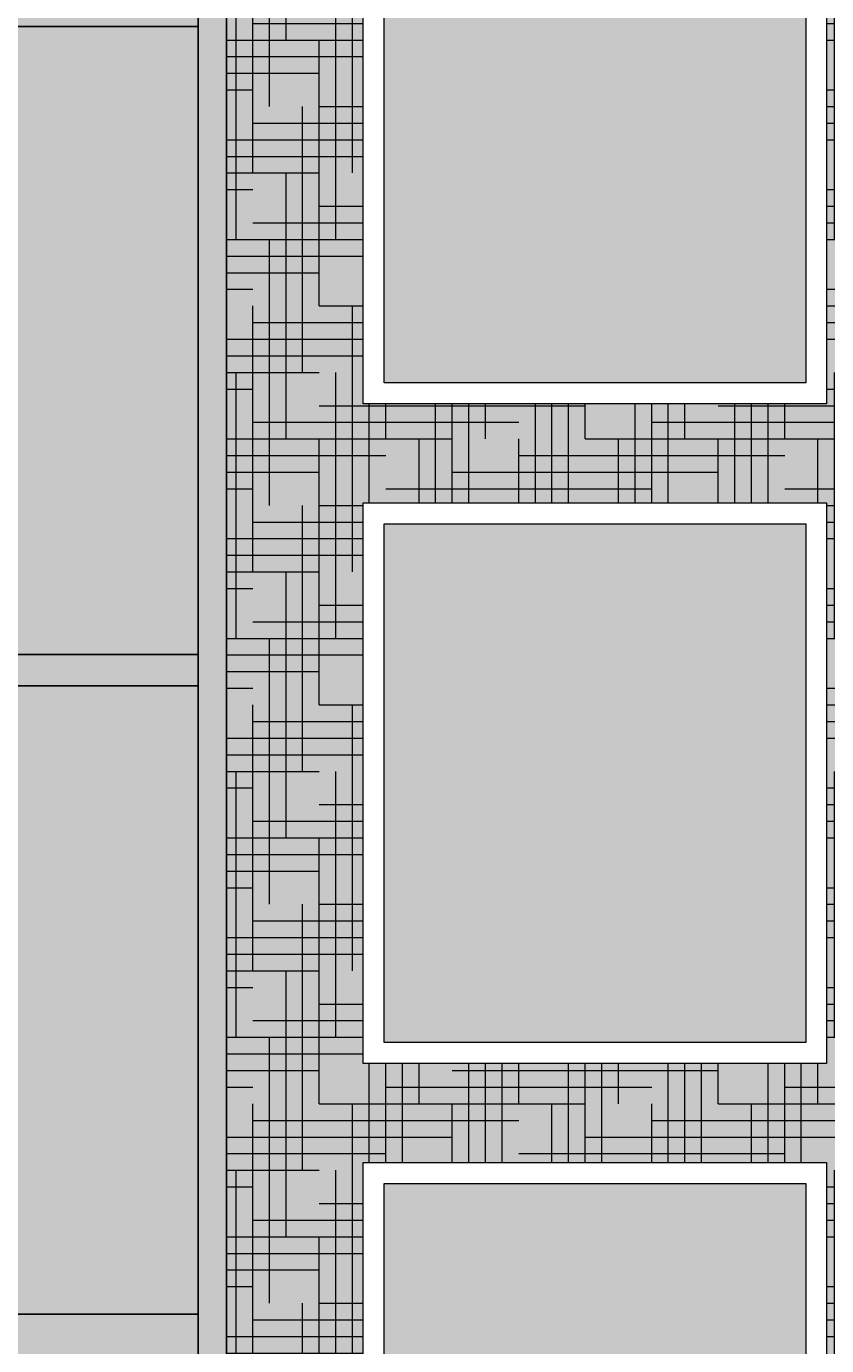
# Model space of a CAD drawing. Units: inches. Extents: x 3024 to 4744, y 1110 to 2100.
# Tile 13 of 29: x 3297 to 3450, y 1402 to 1654. Entities that reach past the tile are written whole.
import ezdxf

# ---------------------------------------------------------------- set-up
doc = ezdxf.new("R2010")
doc.units = ezdxf.units.IN
for name, color, linetype, lineweight in [('A-ANNO-DIMS', 2, 'Continuous', 18), ('A-ELEV', 7, 'Continuous', 25), ('A-ELEV-PATT', 252, 'Continuous', 13), ('A-GLAZ', 4, 'Continuous', 18)]:
    doc.layers.add(name, color=color, linetype=linetype, lineweight=lineweight)
doc.styles.get("Standard").update_dxf_attribs({"font": 'arial.ttf'})
doc.dimstyles.get("Standard").update_dxf_attribs({"dimtxt": 0.18, "dimasz": 0.18, "dimexe": 0.18, "dimexo": 0.0625, "dimgap": 0.09, "dimtad": 0, "dimtih": 1, "dimtoh": 1, "dimdec": 1, "dimzin": 0, "dimdsep": 46, "dimlunit": 3, "dimtxsty": 'Standard', "dimcen": 0.09, "dimadec": 0, "dimazin": 0, "dimtfac": 1, "dimtdec": 1, "dimtofl": 0, "dimtmove": 0, "dimatfit": 3, "dimfxl": 1, "dimtolj": 1, "dimtzin": 0, "dimarcsym": 0})

# ---------------------------------------------------------------- blocks, each defined once
blk = doc.blocks.new('WIN-STONE-CENTRE')
for points in [[(3361.22, 1940.61), (3449.72, 1940.61), (3449.72, 1833.52), (3361.22, 1833.52)], [(3361.22, 1940.61), (3449.72, 1940.61), (3449.72, 1833.52), (3361.22, 1833.52)], [(3365.22, 1936.61), (3445.72, 1936.61), (3445.72, 1837.52), (3365.22, 1837.52)], [(3365.22, 1936.61), (3445.72, 1936.61), (3445.72, 1837.52), (3365.22, 1837.52)]]:
    blk.add_lwpolyline(points, close=True)
blk = doc.blocks.new('*D64')
at = {"layer": 'A-ANNO-DIMS', "color": 0, "lineweight": -2, "transparency": 16777216}
for p, q in [((3069.79, 1241.5), (3069.79, 2100.44)), ((3069.97, 2100.26), (3405.08, 2100.26)), ((3740.97, 2100.26), (3405.87, 2100.26)), ((3741.15, 1241.5), (3741.15, 2100.44))]:
    blk.add_line(p, q, dxfattribs=at)
at = {"layer": 'A-ANNO-DIMS', "color": 0, "transparency": 16777216}
for points in [[(3069.97, 2100.29), (3069.97, 2100.23), (3069.79, 2100.26)], [(3740.97, 2100.29), (3740.97, 2100.23), (3741.15, 2100.26)]]:
    blk.add_solid(points, dxfattribs=at)
at = {"layer": 'Defpoints', "color": 0, "transparency": 16777216}
for p in [(3741.15, 2100.26), (3069.79, 1241.43), (3741.15, 1241.43)]:
    blk.add_point(p, dxfattribs=at)
at = {"layer": 'A-ANNO-DIMS', "color": 0, "transparency": 16777216, "insert": (3405.47, 2100.26), "char_height": 0.18, "attachment_point": 5}
blk.add_mtext('\\A1;671.4', dxfattribs=at)

msp = doc.modelspace()

# ---------------------------------------------------------------- hatches: boundary and pattern name
at = {"layer": 'A-ELEV-PATT'}
h = msp.add_hatch(color=256, dxfattribs=at)
h.dxf.hatch_style = 1
h.paths.add_polyline_path([(3335.1044, 2043.5286), (3329.7033, 2043.5286), (3329.7033, 1155.6112), (3335.1044, 1155.6112)])
h.paths.add_polyline_path([(3481.2411, 2043.5286), (3335.1044, 2043.5286), (3335.1044, 1155.6112), (3481.2411, 1155.6112)])
h.paths.add_polyline_path([(3449.7202, 1329.5246), (3361.2242, 1329.5246), (3361.2242, 1436.6064), (3449.7202, 1436.6064)], flags=16)
h.paths.add_polyline_path([(3445.7202, 1333.5246), (3365.2242, 1333.5246), (3365.2242, 1432.6064), (3445.7202, 1432.6064)], flags=0)
h.paths.add_polyline_path([(3449.7202, 1455.5246), (3361.2242, 1455.5246), (3361.2242, 1562.6064), (3449.7202, 1562.6064)], flags=16)
h.paths.add_polyline_path([(3445.7202, 1459.5246), (3365.2242, 1459.5246), (3365.2242, 1558.6064), (3445.7202, 1558.6064)], flags=0)
h.paths.add_polyline_path([(3449.7202, 1581.5246), (3361.2242, 1581.5246), (3361.2242, 1688.6064), (3449.7202, 1688.6064)], flags=16)
h.paths.add_polyline_path([(3445.7202, 1585.5246), (3365.2242, 1585.5246), (3365.2242, 1684.6064), (3445.7202, 1684.6064)], flags=0)
h.paths.add_polyline_path([(3449.7202, 1707.5246), (3361.2242, 1707.5246), (3361.2242, 1814.6064), (3449.7202, 1814.6064)], flags=16)
h.paths.add_polyline_path([(3445.7202, 1711.5246), (3365.2242, 1711.5246), (3365.2242, 1810.6064), (3445.7202, 1810.6064)], flags=0)
h.paths.add_polyline_path([(3449.7202, 1833.5246), (3361.2242, 1833.5246), (3361.2242, 1940.6064), (3449.7202, 1940.6064)], flags=16)
h.paths.add_polyline_path([(3445.7202, 1837.5246), (3365.2242, 1837.5246), (3365.2242, 1936.6064), (3445.7202, 1936.6064)], flags=0)
h = msp.add_hatch(color=256, dxfattribs=at)
h.dxf.hatch_style = 1
h.paths.add_polyline_path([(3475.84, 2043.5286), (3335.1044, 2043.5286), (3335.1044, 1155.6112), (3475.84, 1155.6112)])
h.paths.add_polyline_path([(3449.7202, 1940.6064), (3449.7202, 1833.5246), (3361.2242, 1833.5246), (3361.2242, 1940.6064)], flags=16)
h.paths.add_polyline_path([(3445.7202, 1936.6064), (3445.7202, 1837.5246), (3365.2242, 1837.5246), (3365.2242, 1936.6064)], flags=0)
h.paths.add_polyline_path([(3449.7202, 1814.6064), (3449.7202, 1707.5246), (3361.2242, 1707.5246), (3361.2242, 1814.6064)], flags=16)
h.paths.add_polyline_path([(3445.7202, 1810.6064), (3445.7202, 1711.5246), (3365.2242, 1711.5246), (3365.2242, 1810.6064)], flags=0)
h.paths.add_polyline_path([(3449.7202, 1688.6064), (3449.7202, 1581.5246), (3361.2242, 1581.5246), (3361.2242, 1688.6064)], flags=16)
h.paths.add_polyline_path([(3445.7202, 1684.6064), (3445.7202, 1585.5246), (3365.2242, 1585.5246), (3365.2242, 1684.6064)], flags=0)
h.paths.add_polyline_path([(3449.7202, 1562.6064), (3449.7202, 1455.5246), (3361.2242, 1455.5246), (3361.2242, 1562.6064)], flags=16)
h.paths.add_polyline_path([(3445.7202, 1558.6064), (3445.7202, 1459.5246), (3365.2242, 1459.5246), (3365.2242, 1558.6064)], flags=0)
h.paths.add_polyline_path([(3449.7202, 1436.6064), (3449.7202, 1329.5246), (3361.2242, 1329.5246), (3361.2242, 1436.6064)], flags=16)
h.paths.add_polyline_path([(3445.7202, 1432.6064), (3445.7202, 1333.5246), (3365.2242, 1333.5246), (3365.2242, 1432.6064)], flags=0)
h = msp.add_hatch(dxfattribs=at)
h.set_pattern_fill('HOUND', color=256, scale=2)
h.paths.add_polyline_path([(3475.84, 2043.5286), (3335.1044, 2043.5286), (3335.1044, 1155.6112), (3475.84, 1155.6112)])
h.paths.add_polyline_path([(3449.7202, 1940.6064), (3449.7202, 1833.5246), (3361.2242, 1833.5246), (3361.2242, 1940.6064)], flags=16)
h.paths.add_polyline_path([(3445.7202, 1936.6064), (3445.7202, 1837.5246), (3365.2242, 1837.5246), (3365.2242, 1936.6064)], flags=0)
h.paths.add_polyline_path([(3449.7202, 1814.6064), (3449.7202, 1707.5246), (3361.2242, 1707.5246), (3361.2242, 1814.6064)], flags=16)
h.paths.add_polyline_path([(3445.7202, 1810.6064), (3445.7202, 1711.5246), (3365.2242, 1711.5246), (3365.2242, 1810.6064)], flags=0)
h.paths.add_polyline_path([(3449.7202, 1688.6064), (3449.7202, 1581.5246), (3361.2242, 1581.5246), (3361.2242, 1688.6064)], flags=16)
h.paths.add_polyline_path([(3445.7202, 1684.6064), (3445.7202, 1585.5246), (3365.2242, 1585.5246), (3365.2242, 1684.6064)], flags=0)
h.paths.add_polyline_path([(3449.7202, 1562.6064), (3449.7202, 1455.5246), (3361.2242, 1455.5246), (3361.2242, 1562.6064)], flags=16)
h.paths.add_polyline_path([(3445.7202, 1558.6064), (3445.7202, 1459.5246), (3365.2242, 1459.5246), (3365.2242, 1558.6064)], flags=0)
h.paths.add_polyline_path([(3449.7202, 1436.6064), (3449.7202, 1329.5246), (3361.2242, 1329.5246), (3361.2242, 1436.6064)], flags=16)
h.paths.add_polyline_path([(3445.7202, 1432.6064), (3445.7202, 1333.5246), (3365.2242, 1333.5246), (3365.2242, 1432.6064)], flags=0)
h = msp.add_hatch(color=256, dxfattribs=at)
h.dxf.hatch_style = 1
h.paths.add_polyline_path([(3445.7202, 1936.6064), (3365.2242, 1936.6064), (3365.2242, 1837.5246), (3445.7202, 1837.5246)])
h.paths.add_polyline_path([(3445.7202, 1810.6064), (3365.2242, 1810.6064), (3365.2242, 1711.5246), (3445.7202, 1711.5246)])
h.paths.add_polyline_path([(3445.7202, 1684.6064), (3365.2242, 1684.6064), (3365.2242, 1585.5246), (3445.7202, 1585.5246)])
h.paths.add_polyline_path([(3445.7202, 1558.6064), (3365.2242, 1558.6064), (3365.2242, 1459.5246), (3445.7202, 1459.5246)])
h.paths.add_polyline_path([(3445.7202, 1432.6064), (3365.2242, 1432.6064), (3365.2242, 1333.5246), (3445.7202, 1333.5246)])
h = msp.add_hatch(color=256, dxfattribs=at)
h.dxf.hatch_style = 1
h.paths.add_polyline_path([(3329.7033, 1407.6112), (3105.4722, 1407.6112), (3105.4722, 1401.6112), (3329.7033, 1401.6112)])
h.paths.add_polyline_path([(3329.7033, 1281.6112), (3105.4722, 1281.6112), (3105.4722, 1275.6112), (3112.3838, 1275.6112), (3329.7033, 1275.6112)])
h.paths.add_polyline_path([(3329.7033, 1533.6112), (3105.4722, 1533.6112), (3105.4722, 1527.6112), (3329.7033, 1527.6112)])
h.paths.add_polyline_path([(3329.7033, 1659.6112), (3105.4722, 1659.6112), (3105.4722, 1653.6112), (3329.7033, 1653.6112)])
h.paths.add_polyline_path([(3329.7033, 1785.6112), (3105.4722, 1785.6112), (3105.4722, 1779.6112), (3329.7033, 1779.6112)])
h.paths.add_polyline_path([(3329.7033, 1911.6112), (3105.4722, 1911.6112), (3095.7158, 1911.6112), (3095.7158, 1905.6112), (3329.7033, 1905.6112)])
h.paths.add_polyline_path([(3715.2286, 1911.6112), (3705.4722, 1911.6112), (3705.4722, 1905.6112), (3715.2286, 1905.6112)])
h.paths.add_polyline_path([(3688.5588, 1911.6112), (3481.2411, 1911.6112), (3481.2411, 1905.6112), (3688.5588, 1905.6112)])
h = msp.add_hatch(color=256, dxfattribs=at)
h.dxf.hatch_style = 1
h.paths.add_polyline_path([(3154.3287, 1897.4879), (3148.9694, 1897.4879), (3148.9694, 1905.6112), (3105.4722, 1905.6112), (3105.4722, 1785.6112), (3148.9694, 1785.6112), (3148.9694, 1795.0431), (3151.6604, 1795.0431), (3151.6604, 1806.8674), (3154.3287, 1806.8674)])
h.paths.add_polyline_path([(3329.7033, 1905.6112), (3292.6051, 1905.6112), (3292.6051, 1897.4879), (3287.2458, 1897.4879), (3287.2458, 1806.8674), (3288.3759, 1806.8674), (3288.3759, 1795.0431), (3292.6051, 1795.0431), (3292.6051, 1785.6112), (3329.7033, 1785.6112)])
h.paths.add_polyline_path([(3154.3287, 1771.4879), (3148.9694, 1771.4879), (3148.9694, 1779.6112), (3105.4722, 1779.6112), (3105.4722, 1659.6112), (3148.9694, 1659.6112), (3148.9694, 1669.0431), (3151.6604, 1669.0431), (3151.6604, 1680.8674), (3154.3287, 1680.8674)])
h.paths.add_polyline_path([(3329.7033, 1779.6112), (3292.6051, 1779.6112), (3292.6051, 1771.4879), (3287.2458, 1771.4879), (3287.2458, 1680.8674), (3288.3759, 1680.8674), (3288.3759, 1669.0431), (3292.6051, 1669.0431), (3292.6051, 1659.6112), (3329.7033, 1659.6112)])
h.paths.add_polyline_path([(3154.3287, 1645.4879), (3148.9694, 1645.4879), (3148.9694, 1653.6112), (3105.4722, 1653.6112), (3105.4722, 1533.6112), (3148.9694, 1533.6112), (3148.9694, 1543.0431), (3151.6604, 1543.0431), (3151.6604, 1554.8674), (3154.3287, 1554.8674)])
h.paths.add_polyline_path([(3329.7033, 1653.6112), (3292.6051, 1653.6112), (3292.6051, 1645.4879), (3287.2458, 1645.4879), (3287.2458, 1554.8674), (3288.3759, 1554.8674), (3288.3759, 1543.0431), (3292.6051, 1543.0431), (3292.6051, 1533.6112), (3329.7033, 1533.6112)])
h.paths.add_polyline_path([(3329.7033, 1527.6112), (3292.6051, 1527.6112), (3292.6051, 1519.4879), (3287.2458, 1519.4879), (3287.2458, 1428.8674), (3288.3759, 1428.8674), (3288.3759, 1417.0431), (3292.6051, 1417.0431), (3292.6051, 1407.6112), (3329.7033, 1407.6112)])
h.paths.add_polyline_path([(3329.7033, 1401.6112), (3292.6051, 1401.6112), (3292.6051, 1393.4879), (3287.2458, 1393.4879), (3287.2458, 1302.8674), (3288.3759, 1302.8674), (3288.3759, 1291.0431), (3292.6051, 1291.0431), (3292.6051, 1281.6112), (3329.7033, 1281.6112)])
h.paths.add_polyline_path([(3154.3287, 1393.4879), (3148.9694, 1393.4879), (3148.9694, 1401.6112), (3105.4722, 1401.6112), (3105.4722, 1281.6112), (3148.9694, 1281.6112), (3148.9694, 1291.0431), (3151.6604, 1291.0431), (3151.6604, 1302.8674), (3154.3287, 1302.8674)])
h.paths.add_polyline_path([(3154.3287, 1519.4879), (3148.9694, 1519.4879), (3148.9694, 1527.6112), (3105.4722, 1527.6112), (3105.4722, 1407.6112), (3148.9694, 1407.6112), (3148.9694, 1417.0431), (3151.6604, 1417.0431), (3151.6604, 1428.8674), (3154.3287, 1428.8674)])
h.paths.add_polyline_path([(3515.7606, 1897.4879), (3510.4013, 1897.4879), (3510.4013, 1905.6112), (3481.2411, 1905.6112), (3481.2411, 1785.6112), (3510.4013, 1785.6112), (3510.4013, 1795.0431), (3513.0923, 1795.0431), (3513.0923, 1806.8674), (3515.7606, 1806.8674)])
h.paths.add_polyline_path([(3688.5588, 1905.6112), (3654.037, 1905.6112), (3654.037, 1897.4879), (3648.6777, 1897.4879), (3648.6777, 1806.8674), (3649.8078, 1806.8674), (3649.8078, 1795.0431), (3654.037, 1795.0431), (3654.037, 1785.6112), (3688.5588, 1785.6112)])
h.paths.add_polyline_path([(3515.7606, 1771.4879), (3510.4013, 1771.4879), (3510.4013, 1779.6112), (3481.2411, 1779.6112), (3481.2411, 1659.6112), (3510.4013, 1659.6112), (3510.4013, 1669.0431), (3513.0923, 1669.0431), (3513.0923, 1680.8674), (3515.7606, 1680.8674)])
h.paths.add_polyline_path([(3688.5588, 1779.6112), (3654.037, 1779.6112), (3654.037, 1771.4879), (3648.6777, 1771.4879), (3648.6777, 1680.8674), (3649.8078, 1680.8674), (3649.8078, 1669.0431), (3654.037, 1669.0431), (3654.037, 1659.6112), (3688.5588, 1659.6112)])
h.paths.add_polyline_path([(3515.7606, 1645.4879), (3510.4013, 1645.4879), (3510.4013, 1653.6112), (3481.2411, 1653.6112), (3481.2411, 1533.6112), (3510.4013, 1533.6112), (3510.4013, 1543.0431), (3513.0923, 1543.0431), (3513.0923, 1554.8674), (3515.7606, 1554.8674)])
h.paths.add_polyline_path([(3688.5588, 1653.6112), (3654.037, 1653.6112), (3654.037, 1645.4879), (3648.6777, 1645.4879), (3648.6777, 1554.8674), (3649.8078, 1554.8674), (3649.8078, 1543.0431), (3654.037, 1543.0431), (3654.037, 1533.6112), (3688.5588, 1533.6112)])
h.paths.add_polyline_path([(3515.7606, 1519.4879), (3510.4013, 1519.4879), (3510.4013, 1527.6112), (3481.2411, 1527.6112), (3481.2411, 1407.6112), (3510.4013, 1407.6112), (3510.4013, 1417.0431), (3513.0923, 1417.0431), (3513.0923, 1428.8674), (3515.7606, 1428.8674)])
h.paths.add_polyline_path([(3688.5588, 1527.6112), (3654.037, 1527.6112), (3654.037, 1519.4879), (3648.6777, 1519.4879), (3648.6777, 1428.8674), (3649.8078, 1428.8674), (3649.8078, 1417.0431), (3654.037, 1417.0431), (3654.037, 1407.6112), (3688.5588, 1407.6112)])
h.paths.add_polyline_path([(3515.7606, 1393.4879), (3510.4013, 1393.4879), (3510.4013, 1401.6112), (3481.2411, 1401.6112), (3481.2411, 1281.6112), (3510.4013, 1281.6112), (3510.4013, 1291.0431), (3513.0923, 1291.0431), (3513.0923, 1302.8674), (3515.7606, 1302.8674)])
h.paths.add_polyline_path([(3688.5588, 1401.6112), (3654.037, 1401.6112), (3654.037, 1393.4879), (3648.6777, 1393.4879), (3648.6777, 1302.8674), (3649.8078, 1302.8674), (3649.8078, 1291.0431), (3654.037, 1291.0431), (3654.037, 1281.6112), (3688.5588, 1281.6112)])
h.paths.add_polyline_path([(3515.7606, 1267.4879), (3510.4013, 1267.4879), (3510.4013, 1275.6112), (3481.2411, 1275.6112), (3481.2411, 1155.6112), (3510.4013, 1155.6112), (3510.4013, 1165.0431), (3513.0923, 1165.0431), (3513.0923, 1176.8674), (3515.7606, 1176.8674)])
h.paths.add_polyline_path([(3688.5588, 1275.6112), (3654.037, 1275.6112), (3654.037, 1267.4879), (3648.6777, 1267.4879), (3648.6777, 1176.8674), (3649.8078, 1176.8674), (3649.8078, 1165.0431), (3654.037, 1165.0431), (3654.037, 1155.6112), (3688.5588, 1155.6112)])
h.paths.add_polyline_path([(3112.3838, 1275.6112), (3105.4722, 1275.6112), (3105.4722, 1171.0239), (3112.3838, 1171.0239)])

# ---------------------------------------------------------------- linework, layer by layer
at = {"layer": 'A-ELEV'}
for p, q in [((3329.7033, 1653.6112), (3105.4722, 1653.6112)), ((3329.7033, 1653.6112), (3105.4722, 1653.6112)), ((3105.4722, 1533.6112), (3329.7033, 1533.6112)), ((3105.4722, 1533.6112), (3329.7033, 1533.6112)), ((3329.7033, 1527.6112), (3105.4722, 1527.6112)), ((3329.7033, 1527.6112), (3105.4722, 1527.6112)), ((3105.4722, 1407.6112), (3329.7033, 1407.6112)), ((3105.4722, 1407.6112), (3329.7033, 1407.6112))]:
    msp.add_line(p, q, dxfattribs=at)
for points in [[(3481.2411, 1155.6112), (3329.7033, 1155.6112), (3329.7033, 2043.5286), (3481.2411, 2043.5286)], [(3329.7033, 2043.5286), (3335.1044, 2043.5286), (3335.1044, 1155.6112), (3329.7033, 1155.6112)], [(3481.2411, 1155.6112), (3329.7033, 1155.6112), (3329.7033, 2043.5286), (3481.2411, 2043.5286)], [(3329.7033, 2043.5286), (3335.1044, 2043.5286), (3335.1044, 1155.6112), (3329.7033, 1155.6112)]]:
    msp.add_lwpolyline(points, close=True, dxfattribs=at)

# ---------------------------------------------------------------- block references
at = {"layer": 'A-GLAZ'}
for p in [(0, -252), (0, -378), (0, -504)]:
    msp.add_blockref('WIN-STONE-CENTRE', p, dxfattribs=at)

# ---------------------------------------------------------------- dimensions: what is measured, and where the dimension line sits
at = {"layer": 'A-ANNO-DIMS'}
dim = msp.add_linear_dim(base=(3741.1507, 2100.2584), p1=(3069.7937, 1241.4341), p2=(3741.1507, 1241.4341), dimstyle='Standard', override={"dimdec": 1, "dimlfac": 1, "dimrnd": 0, "dimzin": 0, "dimdsep": 46, "dimlunit": 2}, dxfattribs=at)
dim.commit()
dim.dimension.update_dxf_attribs({"geometry": '*D64', "text_midpoint": (3405.4722, 2100.2584)})

doc.saveas('drawing.dxf')
